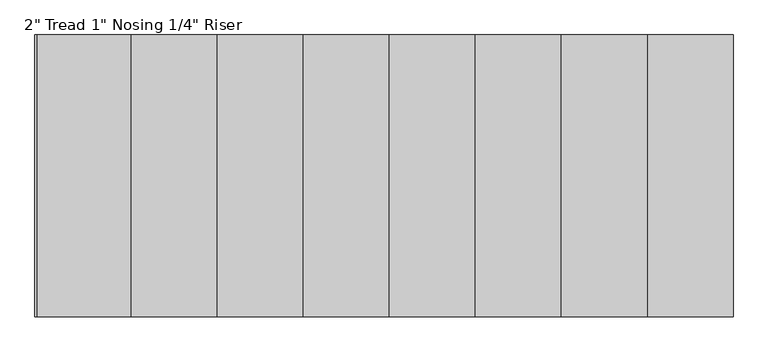
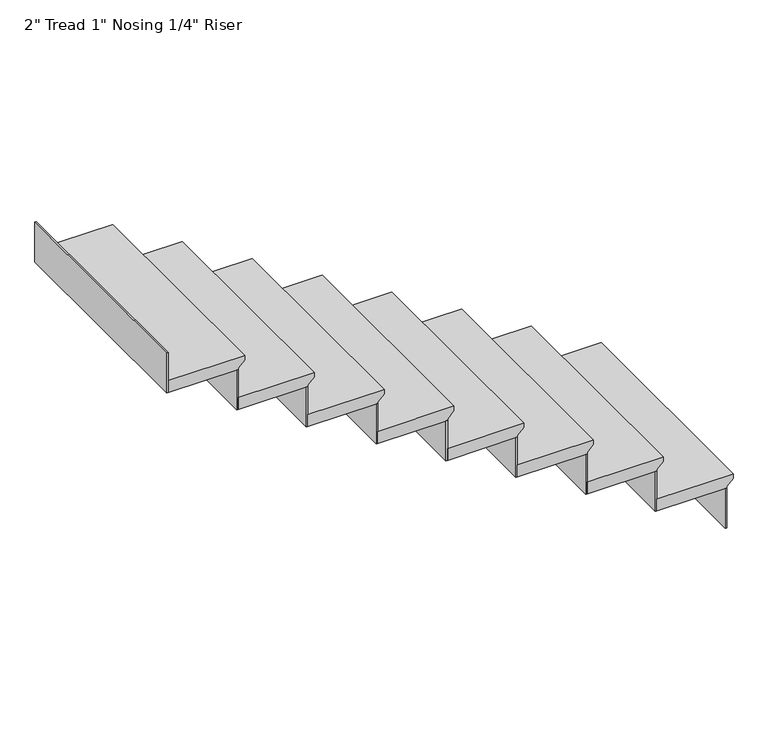
"""IFC4 building model written with IfcOpenShell, lengths in millimetres: stair flight geometry."""

from ifc_helpers import new_model, si_unit, frame, origin, place, context, project, spatial, polyline, outline, extrude, source, transform, mapped, element, save


def stair_flight_e850d810(model_context):
    return source(origin(), model_context, "Body", "SweptSolid", [
        extrude(outline(polyline([(1693.3333333, -1690.2851125), (1693.3333333, -1995.0851125), (1642.5333333, -1995.0851125), (1642.5333333, -1715.6851125), (1648.8833333, -1715.6851125), (1674.2833333, -1690.2851125), (1693.3333333, -1690.2851125)])), frame((0.0, 264.7428815, 0.0), z_axis=(0.0, 1.0, 0.0), x_axis=(0.0, 0.0, 1.0)), (0.0, 0.0, 1.0), 914.4),
        extrude(outline(polyline([(-1722.0351125, 1179.1428815), (-1715.6851125, 1179.1428815), (-1715.6851125, 264.7428815), (-1722.0351125, 264.7428815), (-1722.0351125, 1179.1428815)])), frame((0.0, 0.0, 1473.2), z_axis=(0.0, 0.0, 1.0), x_axis=(1.0, 0.0, 0.0)), (0.0, 0.0, 1.0), 169.3333333),
        extrude(outline(polyline([(-2001.4351125, 1179.1428815), (-1995.0851125, 1179.1428815), (-1995.0851125, 264.7428815), (-2001.4351125, 264.7428815), (-2001.4351125, 1179.1428815)])), frame((0.0, 0.0, 1642.5333333), z_axis=(0.0, 0.0, 1.0), x_axis=(1.0, 0.0, 0.0)), (0.0, 0.0, 1.0), 169.3333333),
        extrude(outline(polyline([(1862.6666667, -1969.6851125), (1862.6666667, -2274.4851125), (1811.8666667, -2274.4851125), (1811.8666667, -1995.0851125), (1818.2166667, -1995.0851125), (1843.6166667, -1969.6851125), (1862.6666667, -1969.6851125)])), frame((0.0, 264.7428815, 0.0), z_axis=(0.0, 1.0, 0.0), x_axis=(0.0, 0.0, 1.0)), (0.0, 0.0, 1.0), 914.4),
        extrude(outline(polyline([(-2280.8351125, 1179.1428815), (-2274.4851125, 1179.1428815), (-2274.4851125, 264.7428815), (-2280.8351125, 264.7428815), (-2280.8351125, 1179.1428815)])), frame((0.0, 0.0, 1811.8666667), z_axis=(0.0, 0.0, 1.0), x_axis=(1.0, 0.0, 0.0)), (0.0, 0.0, 1.0), 169.3333333),
        extrude(outline(polyline([(2032.0, -2249.0851125), (2032.0, -2553.8851125), (1981.2, -2553.8851125), (1981.2, -2274.4851125), (1987.55, -2274.4851125), (2012.95, -2249.0851125), (2032.0, -2249.0851125)])), frame((0.0, 264.7428815, 0.0), z_axis=(0.0, 1.0, 0.0), x_axis=(0.0, 0.0, 1.0)), (0.0, 0.0, 1.0), 914.4),
        extrude(outline(polyline([(-2560.2351125, 1179.1428815), (-2553.8851125, 1179.1428815), (-2553.8851125, 264.7428815), (-2560.2351125, 264.7428815), (-2560.2351125, 1179.1428815)])), frame((0.0, 0.0, 1981.2), z_axis=(0.0, 0.0, 1.0), x_axis=(1.0, 0.0, 0.0)), (0.0, 0.0, 1.0), 169.3333333),
        extrude(outline(polyline([(2201.3333333, -2528.4851125), (2201.3333333, -2833.2851125), (2150.5333333, -2833.2851125), (2150.5333333, -2553.8851125), (2156.8833333, -2553.8851125), (2182.2833333, -2528.4851125), (2201.3333333, -2528.4851125)])), frame((0.0, 264.7428815, 0.0), z_axis=(0.0, 1.0, 0.0), x_axis=(0.0, 0.0, 1.0)), (0.0, 0.0, 1.0), 914.4),
        extrude(outline(polyline([(-2839.6351125, 1179.1428815), (-2833.2851125, 1179.1428815), (-2833.2851125, 264.7428815), (-2839.6351125, 264.7428815), (-2839.6351125, 1179.1428815)])), frame((0.0, 0.0, 2150.5333333), z_axis=(0.0, 0.0, 1.0), x_axis=(1.0, 0.0, 0.0)), (0.0, 0.0, 1.0), 169.3333333),
        extrude(outline(polyline([(2370.6666667, -2807.8851125), (2370.6666667, -3112.6851125), (2319.8666667, -3112.6851125), (2319.8666667, -2833.2851125), (2326.2166667, -2833.2851125), (2351.6166667, -2807.8851125), (2370.6666667, -2807.8851125)])), frame((0.0, 264.7428815, 0.0), z_axis=(0.0, 1.0, 0.0), x_axis=(0.0, 0.0, 1.0)), (0.0, 0.0, 1.0), 914.4),
        extrude(outline(polyline([(-3119.0351125, 1179.1428815), (-3112.6851125, 1179.1428815), (-3112.6851125, 264.7428815), (-3119.0351125, 264.7428815), (-3119.0351125, 1179.1428815)])), frame((0.0, 0.0, 2319.8666667), z_axis=(0.0, 0.0, 1.0), x_axis=(1.0, 0.0, 0.0)), (0.0, 0.0, 1.0), 169.3333333),
        extrude(outline(polyline([(2540.0, -3087.2851125), (2540.0, -3392.0851125), (2489.2, -3392.0851125), (2489.2, -3112.6851125), (2495.55, -3112.6851125), (2520.95, -3087.2851125), (2540.0, -3087.2851125)])), frame((0.0, 264.7428815, 0.0), z_axis=(0.0, 1.0, 0.0), x_axis=(0.0, 0.0, 1.0)), (0.0, 0.0, 1.0), 914.4),
        extrude(outline(polyline([(-3398.4351125, 1179.1428815), (-3392.0851125, 1179.1428815), (-3392.0851125, 264.7428815), (-3398.4351125, 264.7428815), (-3398.4351125, 1179.1428815)])), frame((0.0, 0.0, 2489.2), z_axis=(0.0, 0.0, 1.0), x_axis=(1.0, 0.0, 0.0)), (0.0, 0.0, 1.0), 169.3333333),
        extrude(outline(polyline([(2709.3333333, -3366.6851125), (2709.3333333, -3671.4851125), (2658.5333333, -3671.4851125), (2658.5333333, -3392.0851125), (2664.8833333, -3392.0851125), (2690.2833333, -3366.6851125), (2709.3333333, -3366.6851125)])), frame((0.0, 264.7428815, 0.0), z_axis=(0.0, 1.0, 0.0), x_axis=(0.0, 0.0, 1.0)), (0.0, 0.0, 1.0), 914.4),
        extrude(outline(polyline([(-3677.8351125, 1179.1428815), (-3671.4851125, 1179.1428815), (-3671.4851125, 264.7428815), (-3677.8351125, 264.7428815), (-3677.8351125, 1179.1428815)])), frame((0.0, 0.0, 2658.5333333), z_axis=(0.0, 0.0, 1.0), x_axis=(1.0, 0.0, 0.0)), (0.0, 0.0, 1.0), 169.3333333),
        extrude(outline(polyline([(-3957.2351125, 1179.1428815), (-3950.8851125, 1179.1428815), (-3950.8851125, 264.7428815), (-3957.2351125, 264.7428815), (-3957.2351125, 1179.1428815)])), frame((0.0, 0.0, 2827.8666667), z_axis=(0.0, 0.0, 1.0), x_axis=(1.0, 0.0, 0.0)), (0.0, 0.0, 1.0), 169.3333333),
        extrude(outline(polyline([(2878.6666667, -3646.0851125), (2878.6666667, -3950.8851125), (2827.8666667, -3950.8851125), (2827.8666667, -3671.4851125), (2834.2166667, -3671.4851125), (2859.6166667, -3646.0851125), (2878.6666667, -3646.0851125)])), frame((0.0, 264.7428815, 0.0), z_axis=(0.0, 1.0, 0.0), x_axis=(0.0, 0.0, 1.0)), (0.0, 0.0, 1.0), 914.4),
    ])


if __name__ == "__main__":
    model = new_model("IFC4")
    model_context = context("Model", 3, world=origin())
    ifc_project = project(units=[si_unit("LENGTHUNIT", "METRE", prefix="MILLI")], contexts=[model_context])
    site = spatial("IfcSite", under=ifc_project)
    building = spatial("IfcBuilding", under=site)
    placement = place(None, origin())
    stair_flight_shape = stair_flight_e850d810(model_context)
    element("IfcStairFlight", 1, ObjectType="2\" Tread 1\" Nosing 1/4\" Riser", at=placement, inside=building, context=model_context, shape_type="MappedRepresentation", body=[
        mapped(stair_flight_shape, transform((0.0, 0.0, 0.0), x_axis=(1.0, 0.0, 0.0), y_axis=(0.0, 1.0, 0.0), z_axis=(0.0, 0.0, 1.0))),
    ])
    save(model, "model.ifc")
